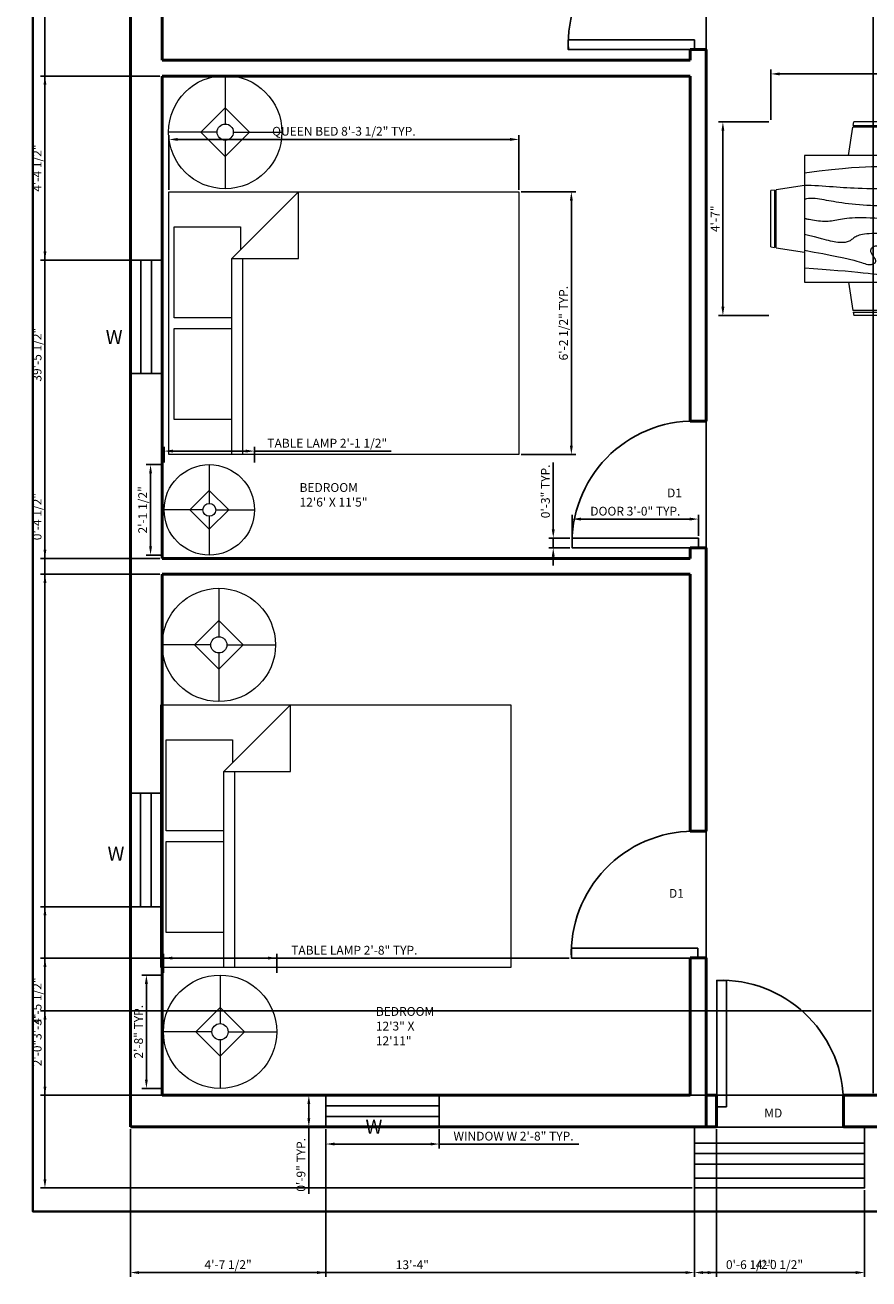
# Model space of a CAD drawing. Units: inches. Extents: x 216 to 622, y 47 to 588.
# Tile 1 of 3: x 216 to 455, y 47 to 403. Entities that reach past the tile are written whole.
import ezdxf

# ---------------------------------------------------------------- set-up
doc = ezdxf.new("R2010")
doc.units = ezdxf.units.IN
for name, color, linetype, lineweight in [('A-ANNO-TTLB', 7, 'Continuous', 35), ('A-AREA-IDEN', 7, 'Continuous', 18), ('A-DOOR', 3, 'Continuous', 25), ('A-FLOR-STRS', 7, 'Continuous', 25), ('A-FURN', 8, 'Continuous', 18), ('A-GLAZ', 4, 'Continuous', 25), ('A-WALL', 7, 'Continuous', 50), ('Dimensions', 1, 'Continuous', 18), ('Text', 6, 'Continuous', 18)]:
    doc.layers.add(name, color=color, linetype=linetype, lineweight=lineweight)
doc.styles.get("Standard").update_dxf_attribs({"font": 'arial.ttf'})
doc.dimstyles.new('ISO-25', dxfattribs={"dimtxt": 2.5, "dimasz": 2.5, "dimexe": 1.25, "dimexo": 0.625, "dimtad": 1, "dimtxsty": 'Standard', "dimcen": 2.5, "dimadec": 0, "dimazin": 0, "dimtfac": 1, "dimtmove": 0, "dimatfit": 3, "dimfxl": 1, "dimarcsym": 0})

# ---------------------------------------------------------------- blocks, each defined once
blk = doc.blocks.new('Dining Set - 36 x 72 in.')
for p, q in [((-22.2343, 26.00059), (-23.4847, 17.99762)), ((-22.2304, 26), (-5.7608, 26)), ((-22, 27.5), (-22.1562, 26.50042)), ((-5.8416, 26.5), (-22.1534, 26.5)), ((-22, 27.5), (-6, 27.5)), ((-5.8437, 26.49966), (-6, 27.5)), ((-4.5152, 17.99762), (-5.7655, 25.99926)), ((5.7657, 26.00059), (4.5153, 17.99762)), ((5.7696, 26), (22.2392, 26)), ((6, 27.5), (5.8438, 26.50042)), ((22.1584, 26.5), (5.8466, 26.5)), ((6, 27.5), (22, 27.5)), ((22.1563, 26.49966), (22, 27.5)), ((23.4848, 17.99762), (22.2345, 25.99926)), ((36, 18), (-36, 18)), ((-36, 18), (-36, -18)), ((36, -18), (36, 18)), ((-45.5, 8), (-44.5004, 8.15617)), ((-45.5, 8), (-45.5, -8)), ((-44.5, -8.15843), (-44.5, 8.15338)), ((-44.0006, 8.23428), (-35.9976, 9.48474)), ((-44, 8.23041), (-44, -8.23915)), ((44.0006, 8.23428), (35.9976, 9.48474)), ((44, 8.23041), (44, -8.23915)), ((44.5, -8.15843), (44.5, 8.15338)), ((45.5, 8), (44.5005, 8.15617)), ((45.5, 8), (45.5, -8)), ((-44.4997, -8.15631), (-45.5, -8)), ((-35.9976, -9.48476), (-43.9993, -8.2345)), ((35.9976, -9.48476), (43.9993, -8.2345)), ((44.4997, -8.15631), (45.5, -8)), ((-36, -18), (36, -18)), ((-22.2343, -26.0006), (-23.4847, -17.99762)), ((-4.5152, -17.99762), (-5.7655, -25.99928)), ((5.7657, -26.0006), (4.5153, -17.99762)), ((23.4848, -17.99762), (22.2345, -25.99928)), ((-22.2304, -26), (-5.7608, -26)), ((-22, -27.5), (-22.1562, -26.50044)), ((-5.8416, -26.5), (-22.1534, -26.5)), ((-22, -27.5), (-6, -27.5)), ((-5.8437, -26.49967), (-6, -27.5)), ((5.7696, -26), (22.2392, -26)), ((6, -27.5), (5.8438, -26.50044)), ((22.1584, -26.5), (5.8466, -26.5)), ((6, -27.5), (22, -27.5)), ((22.1563, -26.49967), (22, -27.5))]:
    blk.add_line(p, q)
for points in [[(-36, 15), (-31.1772, 14.97754), (-26.8079, 14.91406), (-22.8538, 14.81543), (-19.276, 14.6875), (-16.0362, 14.53613), (-13.0957, 14.36718), (-10.4159, 14.18652), (-7.9583, 14), (-5.6904, 13.81315), (-3.6035, 13.63021), (-1.6954, 13.45508), (0.0365, 13.29166), (1.5945, 13.14388), (2.9811, 13.01562), (4.1988, 12.9108), (5.25, 12.83333), (6.1393, 12.78613), (6.8802, 12.76823), (7.4883, 12.77767), (7.9792, 12.8125), (8.3685, 12.87077), (8.6719, 12.95052), (8.9049, 13.0498), (9.0833, 13.16666), (9.2205, 13.29899), (9.3216, 13.44401), (9.3895, 13.59879), (9.4271, 13.76041), (9.4373, 13.92594), (9.4232, 14.09245), (9.3875, 14.257), (9.3333, 14.41666), (9.2638, 14.56917), (9.1836, 14.71484), (9.0975, 14.85465), (9.0104, 14.98958), (8.9272, 15.1206), (8.8529, 15.2487), (8.7922, 15.37483), (8.75, 15.5), (8.7305, 15.62467), (8.7344, 15.74739), (8.7617, 15.86621), (8.8125, 15.97916), (8.8867, 16.08431), (8.9844, 16.17968), (9.1055, 16.26334), (9.25, 16.33333), (9.4189, 16.38802), (9.6172, 16.42708), (9.8506, 16.45052), (10.125, 16.45833), (10.4463, 16.45052), (10.8203, 16.42708), (11.2529, 16.38802), (11.75, 16.33333), (12.3184, 16.26318), (12.9694, 16.17838), (13.7151, 16.07991), (14.5677, 15.96875), (15.5395, 15.84586), (16.6426, 15.71224), (17.8893, 15.56884), (19.2917, 15.41666), (20.859, 15.25667), (22.5879, 15.08984), (24.4721, 14.91715), (26.5052, 14.73958), (28.6809, 14.5581), (30.9929, 14.3737), (33.4347, 14.18733), (36, 14)], [(-36, 10), (-28.9766, 10.14274), (-23.1725, 10.20442), (-18.4241, 10.19775), (-14.5677, 10.13541), (-11.4399, 10.03011), (-8.877, 9.89453), (-6.7154, 9.74137), (-4.7917, 9.58333), (-2.9698, 9.43082), (-1.2246, 9.28515), (0.4415, 9.14534), (2.026, 9.01041), (3.5266, 8.87939), (4.9408, 8.7513), (6.266, 8.62516), (7.5, 8.5), (8.6411, 8.37549), (9.6914, 8.2539), (10.6538, 8.13818), (11.5312, 8.03125), (12.3267, 7.93603), (13.043, 7.85547), (13.6831, 7.79248), (14.25, 7.75), (14.7471, 7.7303), (15.1797, 7.73307), (15.5537, 7.75732), (15.875, 7.80208), (16.1494, 7.86637), (16.3828, 7.94922), (16.5811, 8.04964), (16.75, 8.16666), (16.8944, 8.29915), (17.0143, 8.44531), (17.1089, 8.60319), (17.1771, 8.77083), (17.218, 8.94629), (17.2305, 9.1276), (17.2137, 9.31282), (17.1667, 9.5), (17.0895, 9.6875), (16.987, 9.875), (16.8649, 10.0625), (16.7292, 10.25), (16.5856, 10.4375), (16.4401, 10.625), (16.2985, 10.8125), (16.1667, 11), (16.05, 11.18733), (15.9518, 11.3737), (15.8752, 11.5581), (15.8229, 11.73958), (15.798, 11.91715), (15.8034, 12.08984), (15.842, 12.25667), (15.9167, 12.41666), (16.0295, 12.56836), (16.1784, 12.70833), (16.3605, 12.83268), (16.5729, 12.9375), (16.8127, 13.01888), (17.0768, 13.07291), (17.3625, 13.0957), (17.6667, 13.08333), (17.9894, 13.03312), (18.3418, 12.94726), (18.7382, 12.82918), (19.1927, 12.68229), (19.7195, 12.51001), (20.3327, 12.31575), (21.0465, 12.10294), (21.875, 11.875), (22.8357, 11.63354), (23.959, 11.37304), (25.2786, 11.08618), (26.8282, 10.76562), (28.6414, 10.40405), (30.752, 9.99414), (33.1936, 9.52856), (36, 9)], [(-36, 5.5), (-30.7157, 5.3348), (-26.069, 5.20963), (-21.9946, 5.11767), (-18.4271, 5.05208), (-15.3009, 5.00602), (-12.5508, 4.97265), (-10.1112, 4.94515), (-7.9167, 4.91666), (-5.909, 4.88167), (-4.0586, 4.83984), (-2.3429, 4.79215), (-0.7396, 4.73958), (0.7739, 4.6831), (2.22, 4.6237), (3.6213, 4.56233), (5, 4.5), (6.373, 4.43782), (7.7344, 4.3776), (9.0723, 4.32129), (10.375, 4.27083), (11.6309, 4.22819), (12.8281, 4.19531), (13.9551, 4.17415), (15, 4.16666), (15.954, 4.17448), (16.819, 4.19791), (17.6001, 4.23698), (18.3021, 4.29166), (18.9299, 4.36198), (19.4883, 4.44791), (19.9823, 4.54948), (20.4167, 4.66666), (20.7969, 4.79899), (21.1302, 4.94401), (21.4245, 5.09879), (21.6875, 5.26041), (21.9271, 5.42594), (22.1511, 5.59245), (22.3672, 5.757), (22.5834, 5.91666), (22.8065, 6.06868), (23.0404, 6.21093), (23.2879, 6.34147), (23.5521, 6.45833), (23.8358, 6.55957), (24.142, 6.64323), (24.4735, 6.70735), (24.8334, 6.75), (25.2235, 6.76969), (25.642, 6.76692), (26.0858, 6.74267), (26.5521, 6.69791), (27.0379, 6.63362), (27.5404, 6.55078), (28.0565, 6.45036), (28.5834, 6.33333), (29.1242, 6.19987), (29.7071, 6.04687), (30.3661, 5.87044), (31.1354, 5.66666), (32.0493, 5.43164), (33.142, 5.16146), (34.4475, 4.85221), (36, 4.5)], [(-36, -1), (-30.7915, -0.6591), (-26.0195, -0.38216), (-21.6519, -0.16284), (-17.6563, 0.00521), (-14.0005, 0.12833), (-10.6523, 0.21289), (-7.5796, 0.26522), (-4.75, 0.29166), (-2.134, 0.29793), (0.2878, 0.28711), (2.5317, 0.26163), (4.6146, 0.22396), (6.5529, 0.17651), (8.3633, 0.12174), (10.0623, 0.06209), (11.6667, 0), (13.1899, -0.06201), (14.6341, -0.1211), (15.9982, -0.17432), (17.2813, -0.21875), (18.4823, -0.25147), (19.6003, -0.26953), (20.6343, -0.27002), (21.5834, -0.25), (22.4481, -0.20768), (23.2357, -0.14584), (23.9549, -0.06836), (24.6146, 0.02083), (25.2235, 0.11784), (25.7904, 0.21875), (26.3241, 0.31966), (26.8334, 0.41666), (27.3265, 0.50618), (27.8099, 0.58593), (28.2894, 0.65397), (28.7709, 0.70833), (29.2601, 0.74707), (29.763, 0.76823), (30.2855, 0.76985), (30.8334, 0.75), (31.4088, 0.70784), (31.9994, 0.64713), (32.589, 0.57275), (33.1615, 0.48958), (33.7008, 0.4025), (34.1908, 0.3164), (34.6153, 0.23616), (34.9584, 0.16666), (35.2099, 0.11165), (35.3848, 0.07031), (35.504, 0.04069), (35.5886, 0.02083), (35.6594, 0.00879), (35.7377, 0.0026), (35.8442, 0.00032), (36, 0)], [(-36, -6.5), (-27.1843, -6.31267), (-20.084, -6.1263), (-14.469, -5.9419), (-10.1094, -5.76042), (-6.7752, -5.58285), (-4.2363, -5.41016), (-2.2629, -5.24333), (-0.625, -5.08334), (0.8708, -4.93099), (2.2715, -4.78646), (3.5872, -4.64974), (4.8281, -4.52084), (6.0046, -4.39974), (7.127, -4.28646), (8.2053, -4.18099), (9.25, -4.08334), (10.2705, -3.99382), (11.2734, -3.91407), (12.2647, -3.84603), (13.25, -3.79167), (14.2354, -3.75293), (15.2266, -3.73177), (16.2295, -3.73015), (17.25, -3.75), (18.2912, -3.79248), (19.3451, -3.85547), (20.4009, -3.93604), (21.4479, -4.03125), (22.4754, -4.13819), (23.4727, -4.25391), (24.4289, -4.37549), (25.3334, -4.5), (26.1785, -4.62492), (26.9694, -4.74935), (27.7145, -4.87281), (28.4219, -4.99479), (29.1, -5.11483), (29.7572, -5.23242), (30.4016, -5.34709), (31.0417, -5.45834), (31.6837, -5.56437), (32.3262, -5.65821), (32.9658, -5.73153), (33.599, -5.77604), (34.2224, -5.78345), (34.8327, -5.74545), (35.4264, -5.65373), (36, -5.5)], [(-36, -10), (-26.4022, -9.81299), (-18.4675, -9.62891), (-11.9839, -9.45069), (-6.7396, -9.28125), (-2.5226, -9.12354), (0.8789, -8.98047), (3.6769, -8.85498), (6.0833, -8.75), (8.2767, -8.66765), (10.3021, -8.60677), (12.1712, -8.56543), (13.8958, -8.54167), (15.4876, -8.53353), (16.9583, -8.53907), (18.3197, -8.55632), (19.5834, -8.58334), (20.7616, -8.61841), (21.8685, -8.66081), (22.9188, -8.71004), (23.9271, -8.76563), (24.9081, -8.82707), (25.8763, -8.89388), (26.8465, -8.96558), (27.8334, -9.04167), (28.8474, -9.12118), (29.8828, -9.20117), (30.93, -9.27824), (31.9792, -9.34896), (33.0205, -9.40991), (34.0443, -9.45768), (35.0407, -9.48885), (36, -9.5)], [(-36, -14.5), (-30.0881, -14.33513), (-25.0332, -14.21224), (-20.7312, -14.12647), (-17.0781, -14.07292), (-13.97, -14.04671), (-11.3027, -14.04297), (-8.9724, -14.05681), (-6.875, -14.08334), (-4.9224, -14.11833), (-3.0905, -14.16016), (-1.3709, -14.20785), (0.2448, -14.26042), (1.7647, -14.3169), (3.1973, -14.3763), (4.5507, -14.43767), (5.8333, -14.5), (7.0554, -14.5621), (8.235, -14.62175), (9.3922, -14.67652), (10.5469, -14.72396), (11.7192, -14.76164), (12.929, -14.78711), (14.1965, -14.79794), (15.5417, -14.79167), (16.9933, -14.76424), (18.6152, -14.70508), (20.4804, -14.60197), (22.6615, -14.44271), (25.2312, -14.21509), (28.2624, -13.9069), (31.8277, -13.50594), (36, -13)]]:
    blk.add_lwpolyline(points)
blk = doc.blocks.new('Bed - Queen')
for p, q in [((0, -80.00003), (0, 0)), ((0, 0), (59.99999, 0)), ((59.99999, 0), (59.99999, -80.00003)), ((7.99999, -1.2), (28.79998, -1.2)), ((7.99999, -14.4), (7.99999, -1.2)), ((28.79998, -1.2), (28.79998, -14.4)), ((31.19999, -1.2), (51.99999, -1.2)), ((31.19999, -14.4), (31.19999, -1.2)), ((51.99999, -1.2), (51.99999, -16.4)), ((0, -14.4), (44.8, -14.4)), ((44.8, -16.8), (0, -16.8)), ((59.99999, -29.6), (44.8, -14.4)), ((44.8, -14.4), (44.8, -29.6)), ((51.99999, -16.4), (46.79936, -16.4)), ((44.8, -29.6), (59.99999, -29.6)), ((59.99999, -80.00003), (0, -80.00003))]:
    blk.add_line(p, q)
blk = doc.blocks.new('Lamp - Table')
for p, q in [((0, 7), (0, 1)), ((0, 3), (-3, 0)), ((3, 0), (0, 3)), ((-1, 0), (-7, 0)), ((-3, 0), (0, -3)), ((0, -3), (3, 0)), ((1, 0), (7, 0)), ((0, -1), (0, -7))]:
    blk.add_line(p, q)
for radius in [7, 1]:
    blk.add_circle((0, 0), radius)
blk = doc.blocks.new('WINDOW-W-PLAN')
for p, q in [((0, 0), (0, 32.22)), ((0, 32.22), (9, 32.22)), ((3, 32.22), (3, 0)), ((6, 0), (6, 32.22)), ((9, 32.22), (9, 0)), ((9, 0), (0, 0))]:
    blk.add_line(p, q)
blk = doc.blocks.new('DOOR-PANEL-36IN-NOM')
blk.add_lwpolyline([(35.86, 2.79), (35.86, 0), (0, 0), (0, 2.79)], close=True)
blk = doc.blocks.new('*D15')
at = {"layer": 'Defpoints', "color": 0, "transparency": 16777216}
for p in [(301.07, 90.46), (333.29, 90.46), (333.29, 85.63)]:
    blk.add_point(p, dxfattribs=at)
at = {"layer": 'Dimensions', "color": 0, "lineweight": -2, "transparency": 16777216}
for p, q in [((301.07, 89.84), (301.07, 84.38)), ((333.29, 89.84), (333.29, 84.38)), ((303.57, 85.63), (330.79, 85.63)), ((333.29, 85.63), (372.94, 85.63))]:
    blk.add_line(p, q, dxfattribs=at)
at = {"layer": 'Dimensions', "color": 0, "transparency": 16777216}
for points in [[(303.57, 86.05), (303.57, 85.21), (301.07, 85.63)], [(330.79, 86.05), (330.79, 85.21), (333.29, 85.63)]]:
    blk.add_solid(points, dxfattribs=at)
at = {"layer": 'Dimensions', "color": 0, "transparency": 16777216, "insert": (354.36, 87.55), "char_height": 2.5, "attachment_point": 5}
blk.add_mtext('WINDOW W 2\'-8" TYP.', dxfattribs=at)
blk = doc.blocks.new('*D16')
at = {"layer": 'Defpoints', "color": 0, "transparency": 16777216}
for p in [(301.07, 99.46), (296.23, 90.46), (301.07, 90.46)]:
    blk.add_point(p, dxfattribs=at)
at = {"layer": 'Dimensions', "color": 0, "lineweight": -2, "transparency": 16777216}
for p, q in [((300.44, 99.46), (294.98, 99.46)), ((296.23, 96.96), (296.23, 92.96)), ((300.44, 90.46), (294.98, 90.46)), ((296.23, 90.46), (296.23, 71.48))]:
    blk.add_line(p, q, dxfattribs=at)
at = {"layer": 'Dimensions', "color": 0, "transparency": 16777216}
for points in [[(295.82, 96.96), (296.65, 96.96), (296.23, 99.46)], [(295.82, 92.96), (296.65, 92.96), (296.23, 90.46)]]:
    blk.add_solid(points, dxfattribs=at)
at = {"layer": 'Dimensions', "color": 0, "transparency": 16777216, "insert": (294.33, 79.72), "char_height": 2.5, "attachment_point": 5, "rotation": 90}
blk.add_mtext('0\'-9" TYP.', dxfattribs=at)
blk = doc.blocks.new('*D17')
at = {"layer": 'Defpoints', "color": 0, "transparency": 16777216}
for p in [(280.81, 282.44), (255.13, 278.59), (280.81, 278.59)]:
    blk.add_point(p, dxfattribs=at)
at = {"layer": 'Dimensions', "color": 0, "lineweight": -2, "transparency": 16777216}
for p, q in [((255.13, 279.22), (255.13, 283.69)), ((257.63, 282.44), (278.31, 282.44)), ((280.81, 279.22), (280.81, 283.69)), ((280.81, 282.44), (319.61, 282.44))]:
    blk.add_line(p, q, dxfattribs=at)
at = {"layer": 'Dimensions', "color": 0, "transparency": 16777216}
for points in [[(257.63, 282.86), (257.63, 282.03), (255.13, 282.44)], [(278.31, 282.86), (278.31, 282.03), (280.81, 282.44)]]:
    blk.add_solid(points, dxfattribs=at)
at = {"layer": 'Dimensions', "color": 0, "transparency": 16777216, "insert": (301.46, 284.36), "char_height": 2.5, "attachment_point": 5}
blk.add_mtext('TABLE LAMP 2\'-1 1/2"', dxfattribs=at)
blk = doc.blocks.new('*D18')
at = {"layer": 'Defpoints', "color": 0, "transparency": 16777216}
for p in [(251.28, 278.59), (255.13, 278.59), (255.13, 252.92)]:
    blk.add_point(p, dxfattribs=at)
at = {"layer": 'Dimensions', "color": 0, "lineweight": -2, "transparency": 16777216}
for p, q in [((254.51, 278.59), (250.03, 278.59)), ((251.28, 255.42), (251.28, 276.09)), ((254.51, 252.92), (250.03, 252.92))]:
    blk.add_line(p, q, dxfattribs=at)
at = {"layer": 'Dimensions', "color": 0, "transparency": 16777216}
for points in [[(250.87, 276.09), (251.7, 276.09), (251.28, 278.59)], [(250.87, 255.42), (251.7, 255.42), (251.28, 252.92)]]:
    blk.add_solid(points, dxfattribs=at)
at = {"layer": 'Dimensions', "color": 0, "transparency": 16777216, "insert": (249.37, 265.75), "char_height": 2.5, "attachment_point": 5, "rotation": 90}
blk.add_mtext('2\'-1 1/2"', dxfattribs=at)
blk = doc.blocks.new('*D19')
at = {"layer": 'Defpoints', "color": 0, "transparency": 16777216}
for p in [(287.12, 138.44), (254.93, 133.62), (287.12, 133.62)]:
    blk.add_point(p, dxfattribs=at)
at = {"layer": 'Dimensions', "color": 0, "lineweight": -2, "transparency": 16777216}
for p, q in [((254.93, 134.24), (254.93, 139.69)), ((287.12, 134.24), (287.12, 139.69)), ((257.43, 138.44), (284.62, 138.44)), ((287.12, 138.44), (328.68, 138.44))]:
    blk.add_line(p, q, dxfattribs=at)
at = {"layer": 'Dimensions', "color": 0, "transparency": 16777216}
for points in [[(257.43, 138.86), (257.43, 138.03), (254.93, 138.44)], [(284.62, 138.86), (284.62, 138.03), (287.12, 138.44)]]:
    blk.add_solid(points, dxfattribs=at)
at = {"layer": 'Dimensions', "color": 0, "transparency": 16777216, "insert": (309.15, 140.35), "char_height": 2.5, "attachment_point": 5}
blk.add_mtext('TABLE LAMP 2\'-8" TYP.', dxfattribs=at)
blk = doc.blocks.new('*D20')
at = {"layer": 'Defpoints', "color": 0, "transparency": 16777216}
for p in [(250.1, 133.62), (254.93, 133.62), (254.93, 101.43)]:
    blk.add_point(p, dxfattribs=at)
at = {"layer": 'Dimensions', "color": 0, "lineweight": -2, "transparency": 16777216}
for p, q in [((254.3, 133.62), (248.85, 133.62)), ((250.1, 103.93), (250.1, 131.12)), ((254.3, 101.43), (248.85, 101.43))]:
    blk.add_line(p, q, dxfattribs=at)
at = {"layer": 'Dimensions', "color": 0, "transparency": 16777216}
for points in [[(249.68, 131.12), (250.52, 131.12), (250.1, 133.62)], [(249.68, 103.93), (250.52, 103.93), (250.1, 101.43)]]:
    blk.add_solid(points, dxfattribs=at)
at = {"layer": 'Dimensions', "color": 0, "transparency": 16777216, "insert": (248.2, 117.52), "char_height": 2.5, "attachment_point": 5, "rotation": 90}
blk.add_mtext('2\'-8" TYP.', dxfattribs=at)
blk = doc.blocks.new('*D21')
at = {"layer": 'Defpoints', "color": 0, "transparency": 16777216}
for p in [(406.89, 263.13), (371.03, 257.75), (406.89, 257.75)]:
    blk.add_point(p, dxfattribs=at)
at = {"layer": 'Dimensions', "color": 0, "lineweight": -2, "transparency": 16777216}
for p, q in [((371.03, 258.38), (371.03, 264.38)), ((406.89, 258.38), (406.89, 264.38)), ((373.53, 263.13), (404.39, 263.13))]:
    blk.add_line(p, q, dxfattribs=at)
at = {"layer": 'Dimensions', "color": 0, "transparency": 16777216}
for points in [[(373.53, 263.55), (373.53, 262.71), (371.03, 263.13)], [(404.39, 263.55), (404.39, 262.71), (406.89, 263.13)]]:
    blk.add_solid(points, dxfattribs=at)
at = {"layer": 'Dimensions', "color": 0, "transparency": 16777216, "insert": (388.96, 265.05), "char_height": 2.5, "attachment_point": 5}
blk.add_mtext('DOOR 3\'-0" TYP.', dxfattribs=at)
blk = doc.blocks.new('*D22')
at = {"layer": 'Defpoints', "color": 0, "transparency": 16777216}
for p in [(365.65, 257.75), (371.03, 257.75), (371.03, 254.96)]:
    blk.add_point(p, dxfattribs=at)
at = {"layer": 'Dimensions', "color": 0, "lineweight": -2, "transparency": 16777216}
for p, q in [((365.65, 260.25), (365.65, 279.24)), ((370.4, 257.75), (364.4, 257.75)), ((365.65, 254.96), (365.65, 257.75)), ((370.4, 254.96), (364.4, 254.96)), ((365.65, 252.46), (365.65, 249.96))]:
    blk.add_line(p, q, dxfattribs=at)
at = {"layer": 'Dimensions', "color": 0, "transparency": 16777216}
for points in [[(365.23, 260.25), (366.07, 260.25), (365.65, 257.75)], [(365.23, 252.46), (366.07, 252.46), (365.65, 254.96)]]:
    blk.add_solid(points, dxfattribs=at)
at = {"layer": 'Dimensions', "color": 0, "transparency": 16777216, "insert": (363.75, 271), "char_height": 2.5, "attachment_point": 5, "rotation": 90}
blk.add_mtext('0\'-3" TYP.', dxfattribs=at)
blk = doc.blocks.new('*D25')
at = {"layer": 'Defpoints', "color": 0, "transparency": 16777216}
for p in [(256.48, 370.95), (256.48, 356.04), (355.88, 356.04)]:
    blk.add_point(p, dxfattribs=at)
at = {"layer": 'Dimensions', "color": 0, "lineweight": -2, "transparency": 16777216}
for p, q in [((256.48, 356.67), (256.48, 372.2)), ((353.38, 370.95), (258.98, 370.95)), ((355.88, 356.67), (355.88, 372.2))]:
    blk.add_line(p, q, dxfattribs=at)
at = {"layer": 'Dimensions', "color": 0, "transparency": 16777216}
for points in [[(258.98, 371.37), (258.98, 370.54), (256.48, 370.95)], [(353.38, 371.37), (353.38, 370.54), (355.88, 370.95)]]:
    blk.add_solid(points, dxfattribs=at)
at = {"layer": 'Dimensions', "color": 0, "transparency": 16777216, "insert": (306.18, 372.95), "char_height": 2.5, "attachment_point": 5}
blk.add_mtext('QUEEN BED 8\'-3 1/2" TYP.', dxfattribs=at)
blk = doc.blocks.new('*D26')
at = {"layer": 'Defpoints', "color": 0, "transparency": 16777216}
for p in [(355.88, 356.04), (370.79, 356.04), (355.88, 281.49)]:
    blk.add_point(p, dxfattribs=at)
at = {"layer": 'Dimensions', "color": 0, "lineweight": -2, "transparency": 16777216}
for p, q in [((356.51, 356.04), (372.04, 356.04)), ((370.79, 283.99), (370.79, 353.54)), ((356.51, 281.49), (372.04, 281.49))]:
    blk.add_line(p, q, dxfattribs=at)
at = {"layer": 'Dimensions', "color": 0, "transparency": 16777216}
for points in [[(370.37, 353.54), (371.21, 353.54), (370.79, 356.04)], [(370.37, 283.99), (371.21, 283.99), (370.79, 281.49)]]:
    blk.add_solid(points, dxfattribs=at)
at = {"layer": 'Dimensions', "color": 0, "transparency": 16777216, "insert": (368.87, 318.77), "char_height": 2.5, "attachment_point": 5, "rotation": 90}
blk.add_mtext('6\'-2 1/2" TYP.', dxfattribs=at)
blk = doc.blocks.new('*D37')
at = {"layer": 'Defpoints', "color": 0, "transparency": 16777216}
for p in [(427.48, 389.56), (427.48, 375.91), (518.48, 375.91)]:
    blk.add_point(p, dxfattribs=at)
at = {"layer": 'Dimensions', "color": 0, "lineweight": -2, "transparency": 16777216}
for p, q in [((427.48, 376.53), (427.48, 390.81)), ((515.98, 389.56), (429.98, 389.56)), ((518.48, 376.53), (518.48, 390.81))]:
    blk.add_line(p, q, dxfattribs=at)
at = {"layer": 'Dimensions', "color": 0, "transparency": 16777216}
for points in [[(429.98, 389.98), (429.98, 389.14), (427.48, 389.56)], [(515.98, 389.98), (515.98, 389.14), (518.48, 389.56)]]:
    blk.add_solid(points, dxfattribs=at)
at = {"layer": 'Dimensions', "color": 0, "transparency": 16777216, "insert": (472.98, 391.48), "char_height": 2.5, "attachment_point": 5}
blk.add_mtext('DINING SET 7\'-7"', dxfattribs=at)
blk = doc.blocks.new('*D38')
at = {"layer": 'Defpoints', "color": 0, "transparency": 16777216}
for p in [(427.48, 375.91), (413.83, 320.91), (427.48, 320.91)]:
    blk.add_point(p, dxfattribs=at)
at = {"layer": 'Dimensions', "color": 0, "lineweight": -2, "transparency": 16777216}
for p, q in [((426.85, 375.91), (412.58, 375.91)), ((413.83, 373.41), (413.83, 323.41)), ((426.85, 320.91), (412.58, 320.91))]:
    blk.add_line(p, q, dxfattribs=at)
at = {"layer": 'Dimensions', "color": 0, "transparency": 16777216}
for points in [[(413.41, 373.41), (414.24, 373.41), (413.83, 375.91)], [(413.41, 323.41), (414.24, 323.41), (413.83, 320.91)]]:
    blk.add_solid(points, dxfattribs=at)
at = {"layer": 'Dimensions', "color": 0, "transparency": 16777216, "insert": (411.95, 348.41), "char_height": 2.5, "attachment_point": 5, "rotation": 90}
blk.add_mtext('4\'-7"', dxfattribs=at)
blk = doc.blocks.new('*D45')
at = {"layer": 'Defpoints', "color": 0, "transparency": 16777216}
for p in [(370.82, 138.45), (221.29, 99.47), (404.54, 99.47)]:
    blk.add_point(p, dxfattribs=at)
at = {"layer": 'Dimensions', "color": 0, "lineweight": -2, "transparency": 16777216}
for p, q in [((370.19, 138.45), (220.04, 138.45)), ((221.29, 135.95), (221.29, 101.97)), ((403.91, 99.47), (220.04, 99.47))]:
    blk.add_line(p, q, dxfattribs=at)
at = {"layer": 'Dimensions', "color": 0, "transparency": 16777216}
for points in [[(220.88, 135.95), (221.71, 135.95), (221.29, 138.45)], [(220.88, 101.97), (221.71, 101.97), (221.29, 99.47)]]:
    blk.add_solid(points, dxfattribs=at)
at = {"layer": 'Dimensions', "color": 0, "transparency": 16777216, "insert": (219.39, 118.96), "char_height": 2.5, "attachment_point": 5, "rotation": 90}
blk.add_mtext('3\'-3"', dxfattribs=at)
blk = doc.blocks.new('*D48')
at = {"layer": 'Defpoints', "color": 0, "transparency": 16777216}
for p in [(245.54, 90.47), (301.07, 90.46), (301.07, 49.13)]:
    blk.add_point(p, dxfattribs=at)
at = {"layer": 'Dimensions', "color": 0, "lineweight": -2, "transparency": 16777216}
for p, q in [((245.54, 89.84), (245.54, 47.88)), ((301.07, 89.84), (301.07, 47.88)), ((248.04, 49.13), (298.57, 49.13))]:
    blk.add_line(p, q, dxfattribs=at)
at = {"layer": 'Dimensions', "color": 0, "transparency": 16777216}
for points in [[(248.04, 49.55), (248.04, 48.71), (245.54, 49.13)], [(298.57, 49.55), (298.57, 48.71), (301.07, 49.13)]]:
    blk.add_solid(points, dxfattribs=at)
at = {"layer": 'Dimensions', "color": 0, "transparency": 16777216, "insert": (273.3, 51.05), "char_height": 2.5, "attachment_point": 5}
blk.add_mtext('4\'-7 1/2"', dxfattribs=at)
blk = doc.blocks.new('*D49')
at = {"layer": 'Defpoints', "color": 0, "transparency": 16777216}
for p in [(221.29, 153.04), (254.44, 153.04), (254.54, 99.47)]:
    blk.add_point(p, dxfattribs=at)
at = {"layer": 'Dimensions', "color": 0, "lineweight": -2, "transparency": 16777216}
for p, q in [((253.81, 153.04), (220.04, 153.04)), ((221.29, 101.97), (221.29, 150.54)), ((253.91, 99.47), (220.04, 99.47))]:
    blk.add_line(p, q, dxfattribs=at)
at = {"layer": 'Dimensions', "color": 0, "transparency": 16777216}
for points in [[(220.88, 150.54), (221.71, 150.54), (221.29, 153.04)], [(220.88, 101.97), (221.71, 101.97), (221.29, 99.47)]]:
    blk.add_solid(points, dxfattribs=at)
at = {"layer": 'Dimensions', "color": 0, "transparency": 16777216, "insert": (219.38, 126.25), "char_height": 2.5, "attachment_point": 5, "rotation": 90}
blk.add_mtext('4\'-5 1/2"', dxfattribs=at)
blk = doc.blocks.new('*D50')
at = {"layer": 'Defpoints', "color": 0, "transparency": 16777216}
for p in [(254.54, 388.97), (221.29, 336.66), (254.56, 336.66)]:
    blk.add_point(p, dxfattribs=at)
at = {"layer": 'Dimensions', "color": 0, "lineweight": -2, "transparency": 16777216}
for p, q in [((253.91, 388.97), (220.04, 388.97)), ((221.29, 386.47), (221.29, 339.16)), ((253.93, 336.66), (220.04, 336.66))]:
    blk.add_line(p, q, dxfattribs=at)
at = {"layer": 'Dimensions', "color": 0, "transparency": 16777216}
for points in [[(220.88, 386.47), (221.71, 386.47), (221.29, 388.97)], [(220.88, 339.16), (221.71, 339.16), (221.29, 336.66)]]:
    blk.add_solid(points, dxfattribs=at)
at = {"layer": 'Dimensions', "color": 0, "transparency": 16777216, "insert": (219.38, 362.81), "char_height": 2.5, "attachment_point": 5, "rotation": 90}
blk.add_mtext('4\'-4 1/2"', dxfattribs=at)
blk = doc.blocks.new('*D55')
at = {"layer": 'Defpoints', "color": 0, "transparency": 16777216}
for p in [(405.72, 73.15), (454.06, 73.15), (454.06, 49.13)]:
    blk.add_point(p, dxfattribs=at)
at = {"layer": 'Dimensions', "color": 0, "lineweight": -2, "transparency": 16777216}
for p, q in [((405.72, 72.53), (405.72, 47.88)), ((454.06, 72.53), (454.06, 47.88)), ((408.22, 49.13), (451.56, 49.13))]:
    blk.add_line(p, q, dxfattribs=at)
at = {"layer": 'Dimensions', "color": 0, "transparency": 16777216}
for points in [[(408.22, 49.55), (408.22, 48.71), (405.72, 49.13)], [(451.56, 49.55), (451.56, 48.71), (454.06, 49.13)]]:
    blk.add_solid(points, dxfattribs=at)
at = {"layer": 'Dimensions', "color": 0, "transparency": 16777216, "insert": (429.89, 51.05), "char_height": 2.5, "attachment_point": 5}
blk.add_mtext('4\'-0 1/2"', dxfattribs=at)
blk = doc.blocks.new('*D56')
at = {"layer": 'Defpoints', "color": 0, "transparency": 16777216}
for p in [(245.54, 90.47), (405.72, 90.46), (405.72, 49.13)]:
    blk.add_point(p, dxfattribs=at)
at = {"layer": 'Dimensions', "color": 0, "lineweight": -2, "transparency": 16777216}
for p, q in [((245.54, 89.84), (245.54, 47.88)), ((405.72, 89.84), (405.72, 47.88)), ((248.04, 49.13), (403.22, 49.13))]:
    blk.add_line(p, q, dxfattribs=at)
at = {"layer": 'Dimensions', "color": 0, "transparency": 16777216}
for points in [[(248.04, 49.55), (248.04, 48.71), (245.54, 49.13)], [(403.22, 49.55), (403.22, 48.71), (405.72, 49.13)]]:
    blk.add_solid(points, dxfattribs=at)
at = {"layer": 'Dimensions', "color": 0, "transparency": 16777216, "insert": (325.63, 51.03), "char_height": 2.5, "attachment_point": 5}
blk.add_mtext('13\'-4"', dxfattribs=at)
blk = doc.blocks.new('*D59')
at = {"layer": 'Defpoints', "color": 0, "transparency": 16777216}
for p in [(221.29, 251.97), (254.54, 251.97), (254.54, 247.47)]:
    blk.add_point(p, dxfattribs=at)
at = {"layer": 'Dimensions', "color": 0, "lineweight": -2, "transparency": 16777216}
for p, q in [((221.29, 254.47), (221.29, 270.69)), ((253.91, 251.97), (220.04, 251.97)), ((221.29, 247.47), (221.29, 251.97)), ((253.91, 247.47), (220.04, 247.47)), ((221.29, 244.97), (221.29, 242.47))]:
    blk.add_line(p, q, dxfattribs=at)
at = {"layer": 'Dimensions', "color": 0, "transparency": 16777216}
for points in [[(220.88, 254.47), (221.71, 254.47), (221.29, 251.97)], [(220.88, 244.97), (221.71, 244.97), (221.29, 247.47)]]:
    blk.add_solid(points, dxfattribs=at)
at = {"layer": 'Dimensions', "color": 0, "transparency": 16777216, "insert": (219.38, 263.83), "char_height": 2.5, "attachment_point": 5, "rotation": 90}
blk.add_mtext('0\'-4 1/2"', dxfattribs=at)
blk = doc.blocks.new('*D61')
at = {"layer": 'Defpoints', "color": 0, "transparency": 16777216}
for p in [(221.29, 123.47), (456.54, 123.47), (456.54, 99.47)]:
    blk.add_point(p, dxfattribs=at)
at = {"layer": 'Dimensions', "color": 0, "lineweight": -2, "transparency": 16777216}
for p, q in [((455.91, 123.47), (220.04, 123.47)), ((221.29, 101.97), (221.29, 120.97)), ((455.91, 99.47), (220.04, 99.47))]:
    blk.add_line(p, q, dxfattribs=at)
at = {"layer": 'Dimensions', "color": 0, "transparency": 16777216}
for points in [[(220.88, 120.97), (221.71, 120.97), (221.29, 123.47)], [(220.88, 101.97), (221.71, 101.97), (221.29, 99.47)]]:
    blk.add_solid(points, dxfattribs=at)
at = {"layer": 'Dimensions', "color": 0, "transparency": 16777216, "insert": (219.39, 111.47), "char_height": 2.5, "attachment_point": 5, "rotation": 90}
blk.add_mtext('2\'-0"', dxfattribs=at)
blk = doc.blocks.new('*D62')
at = {"layer": 'Defpoints', "color": 0, "transparency": 16777216}
for p in [(456.54, 570.49), (409.04, 99.47), (456.54, 99.47)]:
    blk.add_point(p, dxfattribs=at)
at = {"layer": 'Dimensions', "color": 0, "lineweight": -2, "transparency": 16777216}
for p, q in [((409.04, 100.09), (409.04, 571.74)), ((411.54, 570.49), (454.04, 570.49)), ((456.54, 100.09), (456.54, 571.74))]:
    blk.add_line(p, q, dxfattribs=at)
at = {"layer": 'Dimensions', "color": 0, "transparency": 16777216}
for points in [[(411.54, 570.9), (411.54, 570.07), (409.04, 570.49)], [(454.04, 570.9), (454.04, 570.07), (456.54, 570.49)]]:
    blk.add_solid(points, dxfattribs=at)
at = {"layer": 'Dimensions', "color": 0, "transparency": 16777216, "insert": (432.79, 572.4), "char_height": 2.5, "attachment_point": 5}
blk.add_mtext('3\'-11 1/2"', dxfattribs=at)
blk = doc.blocks.new('*D64')
at = {"layer": 'Defpoints', "color": 0, "transparency": 16777216}
for p in [(221.29, 546.47), (245.54, 546.47), (405.72, 73.15)]:
    blk.add_point(p, dxfattribs=at)
at = {"layer": 'Dimensions', "color": 0, "lineweight": -2, "transparency": 16777216}
for p, q in [((244.91, 546.47), (220.04, 546.47)), ((221.29, 75.65), (221.29, 543.97)), ((405.09, 73.15), (220.04, 73.15))]:
    blk.add_line(p, q, dxfattribs=at)
at = {"layer": 'Dimensions', "color": 0, "transparency": 16777216}
for points in [[(220.88, 543.97), (221.71, 543.97), (221.29, 546.47)], [(220.88, 75.65), (221.71, 75.65), (221.29, 73.15)]]:
    blk.add_solid(points, dxfattribs=at)
at = {"layer": 'Dimensions', "color": 0, "transparency": 16777216, "insert": (219.37, 309.81), "char_height": 2.5, "attachment_point": 5, "rotation": 90}
blk.add_mtext('39\'-5 1/2"', dxfattribs=at)
blk = doc.blocks.new('*D68')
at = {"layer": 'Defpoints', "color": 0, "transparency": 16777216}
for p in [(405.72, 90.46), (412.04, 90.47), (412.04, 49.13)]:
    blk.add_point(p, dxfattribs=at)
at = {"layer": 'Dimensions', "color": 0, "lineweight": -2, "transparency": 16777216}
for p, q in [((405.72, 89.84), (405.72, 47.88)), ((412.04, 89.84), (412.04, 47.88)), ((408.22, 49.13), (409.54, 49.13)), ((412.04, 49.13), (428.26, 49.13))]:
    blk.add_line(p, q, dxfattribs=at)
at = {"layer": 'Dimensions', "color": 0, "transparency": 16777216}
for points in [[(408.22, 49.55), (408.22, 48.71), (405.72, 49.13)], [(409.54, 49.55), (409.54, 48.71), (412.04, 49.13)]]:
    blk.add_solid(points, dxfattribs=at)
at = {"layer": 'Dimensions', "color": 0, "transparency": 16777216, "insert": (421.4, 51.05), "char_height": 2.5, "attachment_point": 5}
blk.add_mtext('0\'-6 1/2"', dxfattribs=at)

msp = doc.modelspace()

# ---------------------------------------------------------------- linework, layer by layer
at = {"layer": 'A-ANNO-TTLB'}
msp.add_lwpolyline([(217.87, 587.77), (621.96, 587.77), (621.96, 66.45), (217.87, 66.45)], close=True, dxfattribs=at)
at = {"layer": 'A-DOOR'}
for centre, radius, start, end in [((402.83, 398.09), 32.93, 86.4001, 182.8834), ((405.61, 256.35), 34.63, 89.4114, 182.3078), ((405.57, 139.69), 34.79, 90.5278, 182.0478), ((413.33, 97.4), 34.73, 2.1734, 92.0276)]:
    msp.add_arc(centre, radius, start, end, dxfattribs=at)
at = {"layer": 'A-FLOR-STRS'}
for p, q in [((454.06, 85.92), (405.72, 85.92)), ((454.06, 82.92), (405.72, 82.92)), ((454.06, 79.92), (405.72, 79.92)), ((454.06, 75.92), (405.72, 75.92))]:
    msp.add_line(p, q, dxfattribs=at)
msp.add_lwpolyline([(405.72, 90.46), (454.06, 90.46), (454.06, 73.15), (405.72, 73.15)], close=True, dxfattribs=at)
at = {"layer": 'A-WALL'}
for p, q in [((245.54, 90.47), (245.54, 546.47)), ((254.54, 393.47), (254.54, 537.47)), ((404.54, 393.47), (404.54, 396.47)), ((404.54, 396.47), (409.04, 396.47)), ((404.54, 393.47), (404.54, 396.47)), ((409.04, 388.97), (409.04, 396.47)), ((409.04, 290.97), (409.04, 396.47)), ((254.54, 393.47), (404.54, 393.47)), ((254.54, 388.97), (404.54, 388.97)), ((254.54, 251.97), (254.54, 388.97)), ((404.54, 290.97), (404.54, 388.97)), ((404.54, 290.97), (409.04, 290.97)), ((404.54, 254.97), (409.04, 254.97)), ((404.54, 251.97), (404.54, 254.97)), ((409.04, 174.47), (409.04, 254.97)), ((254.54, 251.97), (404.54, 251.97)), ((254.54, 99.47), (254.54, 247.47)), ((254.54, 247.47), (404.54, 247.47)), ((404.54, 174.47), (404.54, 247.47)), ((409.04, 174.47), (404.54, 174.47)), ((404.54, 99.47), (404.54, 138.47)), ((409.04, 138.47), (404.54, 138.47)), ((409.04, 90.47), (409.04, 138.47)), ((404.54, 99.47), (254.54, 99.47)), ((412.04, 99.47), (409.04, 99.47)), ((412.04, 90.47), (412.04, 99.47)), ((572.54, 99.47), (448.04, 99.47)), ((448.04, 90.47), (448.04, 99.47)), ((412.04, 90.47), (245.54, 90.47)), ((581.54, 90.47), (448.04, 90.47))]:
    msp.add_line(p, q, dxfattribs=at)

# ---------------------------------------------------------------- block references
at = {"layer": 'A-DOOR'}
for p in [(369.93, 396.46), (371.03, 254.96), (370.82, 138.45)]:
    msp.add_blockref('DOOR-PANEL-36IN-NOM', p, dxfattribs=at)
at = {"layer": 'A-DOOR', "rotation": 269.9999999999999}
msp.add_blockref('DOOR-PANEL-36IN-NOM', (412.1, 132.1), dxfattribs=at)
at = {"layer": 'A-FURN'}
for p, xscale, yscale, zscale in [((272.49, 373.03), 2.299024098102729, 2.299024098102729, 2.299024098102729), ((267.97, 265.75), 1.833899009384919, 1.833899009384919, 1.833899009384919), ((270.68, 227.4), 2.299024098102729, 2.299024098102729, 2.299024098102729), ((271.02, 117.52), 2.299024098102729, 2.299024098102729, 2.299024098102729)]:
    msp.add_blockref('Lamp - Table', p, dxfattribs=dict(at, xscale=xscale, yscale=yscale, zscale=zscale))
at = {"layer": 'A-FURN', "rotation": 180}
msp.add_blockref('Dining Set - 36 x 72 in.', (472.98, 348.41), dxfattribs=at)
at = {"layer": 'A-FURN', "xscale": 1.242515159036098, "yscale": 1.242515159036098, "zscale": 1.242515159036098, "rotation": 90}
for p in [(256.48, 281.49), (254.21, 135.81)]:
    msp.add_blockref('Bed - Queen', p, dxfattribs=at)
at = {"layer": 'A-GLAZ'}
for p, rotation in [((254.56, 336.65), 180), ((254.44, 185.26), 180), ((301.07, 99.46), 270)]:
    msp.add_blockref('WINDOW-W-PLAN', p, dxfattribs=dict(at, rotation=rotation))

# ---------------------------------------------------------------- texts
at = {"layer": 'A-AREA-IDEN', "char_height": 2.5, "attachment_point": 1}
for s, width, insert in [('BEDROOM\\P12\'6\' X 11\'5"', 53.9506, (293.59, 273.35)), ('BEDROOM\\P12\'3" X 12\'11"', 21.6971, (315.26, 124.54))]:
    msp.add_mtext_dynamic_manual_height_columns(s, width=width, gutter_width=12.5, heights=[0], dxfattribs=dict(at, insert=insert))
at = {"layer": 'Text', "attachment_point": 1}
for s, width, gutter_width, insert, char_height in [('W', 20.8525, 20.07, (238.54, 316.86), 4.01), ('D1', 14.8305, 12.5, (397.97, 271.81), 2.5), ('W', 20.8525, 20.07, (239.06, 170.13), 4.01), ('D1 ', 11.0272, 12.5, (398.51, 158.08), 2.5), ('MD', 2.407, 12.5, (425.58, 95.68), 2.5), ('W', 20.8525, 20.07, (312.32, 92.57), 4.01)]:
    msp.add_mtext_dynamic_manual_height_columns(s, width=width, gutter_width=gutter_width, heights=[0], dxfattribs=dict(at, insert=insert, char_height=char_height))

# ---------------------------------------------------------------- dimensions: what is measured, and where the dimension line sits
at = {"layer": 'Dimensions'}
for base, p1, p2, picture, middle in [((456.54, 570.49), (409.04, 99.47), (456.54, 99.47), '*D62', (432.79, 572.4)), ((301.07, 49.13), (245.54, 90.47), (301.07, 90.46), '*D48', (273.3, 51.05)), ((405.72, 49.13), (245.54, 90.47), (405.72, 90.46), '*D56', (325.63, 51.03)), ((412.04, 49.13), (405.72, 90.46), (412.04, 90.47), '*D68', (421.4, 51.05)), ((454.06, 49.13), (405.72, 73.15), (454.06, 73.15), '*D55', (429.89, 51.05))]:
    dim = msp.add_linear_dim(base=base, p1=p1, p2=p2, dimstyle='ISO-25', override={"dimdec": 1, "dimlfac": 1, "dimrnd": 0, "dimzin": 1, "dimdsep": 46, "dimlunit": 4, "dimfrac": 2}, dxfattribs=at)
    dim.commit()
    dim.dimension.update_dxf_attribs({"geometry": picture, "text_midpoint": middle})
for base, p1, p2, angle, picture, middle in [((221.29, 546.47), (405.72, 73.15), (245.54, 546.47), 90, '*D64', (219.37, 309.81)), ((221.29, 336.66), (254.54, 388.97), (254.56, 336.66), 90, '*D50', (219.38, 362.81)), ((413.83, 320.91), (427.48, 375.91), (427.48, 320.91), 270, '*D38', (411.95, 348.41)), ((251.28, 278.59), (255.13, 252.92), (255.13, 278.59), 90, '*D18', (249.37, 265.75)), ((221.29, 251.97), (254.54, 247.47), (254.54, 251.97), 90, '*D59', (219.38, 263.83)), ((221.29, 153.04), (254.54, 99.47), (254.44, 153.04), 90, '*D49', (219.38, 126.25)), ((221.29, 99.47), (370.82, 138.45), (404.54, 99.47), 90, '*D45', (219.39, 118.96)), ((221.29, 123.47), (456.54, 99.47), (456.54, 123.47), 90, '*D61', (219.39, 111.47))]:
    dim = msp.add_linear_dim(base=base, p1=p1, p2=p2, angle=angle, dimstyle='ISO-25', override={"dimdec": 1, "dimlfac": 1, "dimrnd": 0, "dimzin": 1, "dimdsep": 46, "dimlunit": 4, "dimfrac": 2}, dxfattribs=at)
    dim.commit()
    dim.dimension.update_dxf_attribs({"geometry": picture, "text_midpoint": middle})
for base, p1, p2, angle, text, picture, middle in [((427.48, 389.56), (518.48, 375.91), (427.48, 375.91), 180, 'DINING SET <>', '*D37', (472.98, 391.48)), ((256.48, 370.95), (355.88, 356.04), (256.48, 356.04), 180, 'QUEEN BED <> TYP.', '*D25', (306.18, 372.95)), ((370.7908, 356.0425), (355.8806, 281.4916), (355.8806, 356.0425), 90, '<> TYP.', '*D26', (368.8732, 318.7671)), ((365.65, 257.75), (371.03, 254.96), (371.03, 257.75), 90, '<> TYP.', '*D22', (363.75, 271)), ((250.1, 133.62), (254.93, 101.43), (254.93, 133.62), 90, '<> TYP.', '*D20', (248.2, 117.52)), ((296.23, 90.46), (301.07, 99.46), (301.07, 90.46), 270, '<> TYP.', '*D16', (294.33, 79.72))]:
    dim = msp.add_linear_dim(base=base, p1=p1, p2=p2, angle=angle, text=text, dimstyle='ISO-25', override={"dimdec": 1, "dimlfac": 1, "dimrnd": 0, "dimzin": 1, "dimdsep": 46, "dimlunit": 4, "dimfrac": 2}, dxfattribs=at)
    dim.commit()
    dim.dimension.update_dxf_attribs({"geometry": picture, "text_midpoint": middle})
for base, p1, p2, text, picture, middle in [((280.81, 282.44), (255.13, 278.59), (280.81, 278.59), 'TABLE LAMP <>', '*D17', (301.46, 284.36)), ((406.89, 263.13), (371.03, 257.75), (406.89, 257.75), 'DOOR <> TYP.', '*D21', (388.96, 265.05)), ((287.12, 138.44), (254.93, 133.62), (287.12, 133.62), 'TABLE LAMP <> TYP.', '*D19', (309.15, 140.35)), ((333.29, 85.63), (301.07, 90.46), (333.29, 90.46), 'WINDOW W <> TYP.', '*D15', (354.36, 87.55))]:
    dim = msp.add_linear_dim(base=base, p1=p1, p2=p2, text=text, dimstyle='ISO-25', override={"dimdec": 1, "dimlfac": 1, "dimrnd": 0, "dimzin": 1, "dimdsep": 46, "dimlunit": 4, "dimfrac": 2}, dxfattribs=at)
    dim.commit()
    dim.dimension.update_dxf_attribs({"geometry": picture, "text_midpoint": middle})

doc.saveas('drawing.dxf')
